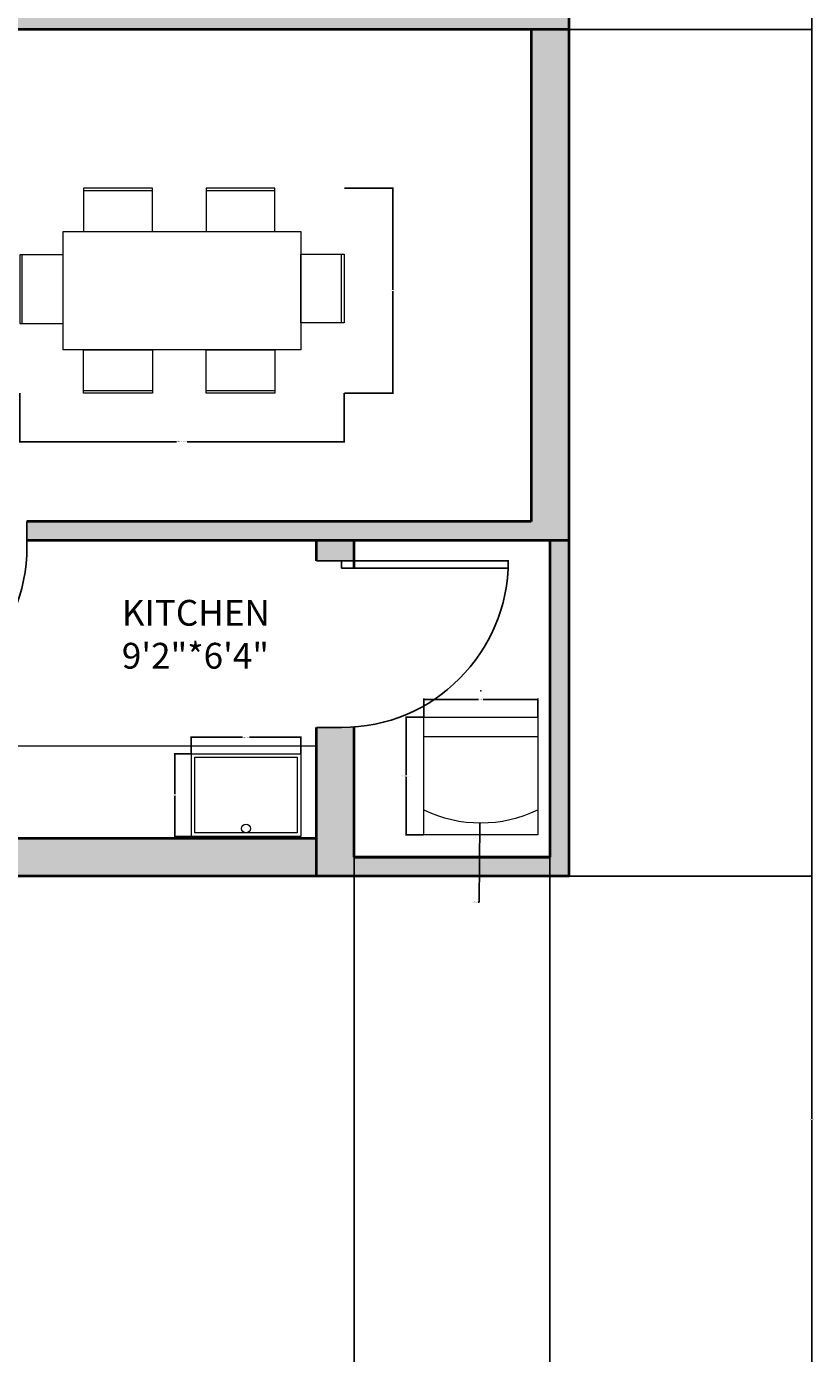
# Model space of a CAD drawing. Units: inches. Extents: x 1642 to 2399, y 1011 to 2291.
# Tile 6 of 7: x 2210 to 2399, y 1595 to 1913. Entities that reach past the tile are written whole.
import ezdxf

# ---------------------------------------------------------------- set-up
doc = ezdxf.new("R2010")
doc.units = ezdxf.units.IN
for name, color, linetype, lineweight in [('A-ANNO-DIMS', 2, 'Continuous', 18), ('A-AREA-IDEN', 7, 'Continuous', 20), ('A-DOOR', 4, 'Continuous', 25), ('A-EQPM', 8, 'Continuous', 18), ('A-FLOR-CASE', 30, 'Continuous', 18), ('A-FLOR-FIXT', 9, 'Continuous', 18), ('A-FURN', 8, 'Continuous', 18), ('A-WALL-PATT', 40, 'Continuous', 13), ('WALL', 40, 'Continuous', 40)]:
    doc.layers.add(name, color=color, linetype=linetype, lineweight=lineweight)
doc.styles.get("Standard").update_dxf_attribs({"font": 'arial.ttf'})
doc.dimstyles.get("Standard").update_dxf_attribs({"dimtxt": 0.18, "dimasz": 0.18, "dimexe": 0.18, "dimexo": 0.0625, "dimgap": 0.09, "dimtad": 0, "dimtih": 1, "dimtoh": 1, "dimdec": 4, "dimzin": 0, "dimdsep": 46, "dimtxsty": 'Standard', "dimcen": 0.09, "dimadec": 0, "dimazin": 0, "dimtfac": 1, "dimtdec": 4, "dimtofl": 0, "dimtmove": 0, "dimatfit": 3, "dimfxl": 1, "dimtolj": 1, "dimtzin": 0, "dimarcsym": 0})

# ---------------------------------------------------------------- blocks, each defined once
blk = doc.blocks.new('*U2')
for p, q in [((0, 0), (0, -6)), ((40, 0), (40, -6))]:
    blk.add_line(p, q)
blk.add_lwpolyline([(0, 0), (0, 40), (1.75, 40), (1.75, 0)], close=True)
blk.add_arc((0, 0), 40, 0, 90)
blk = doc.blocks.new('TABLE-DINING-SIX-SEAT')
for p, q in [((15.31, 48.55), (31.81, 48.55)), ((44.68, 48.55), (61.18, 48.55)), ((0.59, 16.67), (0.59, 33.17)), ((77.22, 16.83), (77.22, 33.33)), ((15.31, 0.59), (31.81, 0.59)), ((44.68, 0.59), (61.18, 0.59))]:
    blk.add_line(p, q)
for points in [[(15.31, 38.77), (31.81, 38.77), (31.81, 49.15), (15.31, 49.15)], [(44.68, 38.77), (61.18, 38.77), (61.18, 49.15), (44.68, 49.15)], [(10.38, 38.77), (67.43, 38.77), (67.43, 10.38), (10.38, 10.38)], [(10.38, 16.67), (10.38, 33.17), (0, 33.17), (0, 16.67)], [(67.43, 16.83), (67.43, 33.33), (77.81, 33.33), (77.81, 16.83)], [(15.31, 10.38), (31.81, 10.38), (31.81, 0), (15.31, 0)], [(44.68, 10.38), (61.18, 10.38), (61.18, 0), (44.68, 0)]]:
    blk.add_lwpolyline(points, close=True)
blk = doc.blocks.new('SINK-KITCHEN-SINGLE')
for points in [[(0, 19.82), (26.24, 19.82), (26.24, 0), (0, 0)], [(0.83, 18.98), (25.41, 18.98), (25.41, 0.83), (0.83, 0.83)]]:
    blk.add_lwpolyline(points, close=True)
blk.add_circle((13.12, 17.93), 1.05)
blk = doc.blocks.new('UTILITY-APPLIANCE')
blk.add_line((0, 4.7), (27.35, 4.7))
blk.add_lwpolyline([(0, 28.26), (27.35, 28.26), (27.35, 0), (0, 0)], close=True)
blk.add_arc((13.68, -6.28), 31.65, 64.3994, 115.6006)
blk = doc.blocks.new('*D18')
at = {"layer": 'A-ANNO-DIMS', "color": 0, "lineweight": -2, "transparency": 16777216}
for p, q in [((2208.46, 1825.25), (2208.46, 1813.46)), ((2286.28, 1825.25), (2286.28, 1813.46)), ((2208.64, 1813.64), (2246.09, 1813.64)), ((2286.1, 1813.64), (2248.65, 1813.64))]:
    blk.add_line(p, q, dxfattribs=at)
at = {"layer": 'A-ANNO-DIMS', "color": 0, "transparency": 16777216}
for points in [[(2208.64, 1813.67), (2208.64, 1813.61), (2208.46, 1813.64)], [(2286.1, 1813.67), (2286.1, 1813.61), (2286.28, 1813.64)]]:
    blk.add_solid(points, dxfattribs=at)
at = {"layer": 'Defpoints', "color": 0, "transparency": 16777216}
for p in [(2208.46, 1825.31), (2286.28, 1825.31), (2286.28, 1813.64)]:
    blk.add_point(p, dxfattribs=at)
at = {"layer": 'A-ANNO-DIMS', "color": 0, "transparency": 16777216, "insert": (2247.37, 1813.64), "char_height": 0.18, "attachment_point": 5}
blk.add_mtext('\\A1;DINING SET 78 TYP.', dxfattribs=at)
blk = doc.blocks.new('*D19')
at = {"layer": 'A-ANNO-DIMS', "color": 0, "lineweight": -2, "transparency": 16777216}
for p, q in [((2286.34, 1874.46), (2298.13, 1874.46)), ((2297.95, 1874.28), (2297.95, 1850.07)), ((2297.95, 1825.49), (2297.95, 1849.7)), ((2286.34, 1825.31), (2298.13, 1825.31))]:
    blk.add_line(p, q, dxfattribs=at)
at = {"layer": 'A-ANNO-DIMS', "color": 0, "transparency": 16777216}
for points in [[(2297.92, 1874.28), (2297.98, 1874.28), (2297.95, 1874.46)], [(2297.92, 1825.49), (2297.98, 1825.49), (2297.95, 1825.31)]]:
    blk.add_solid(points, dxfattribs=at)
at = {"layer": 'Defpoints', "color": 0, "transparency": 16777216}
for p in [(2286.28, 1874.46), (2297.95, 1874.46), (2286.28, 1825.31)]:
    blk.add_point(p, dxfattribs=at)
at = {"layer": 'A-ANNO-DIMS', "color": 0, "transparency": 16777216, "insert": (2297.95, 1849.88), "char_height": 0.18, "attachment_point": 5}
blk.add_mtext('\\A1;49 TYP.', dxfattribs=at)
blk = doc.blocks.new('*D24')
at = {"layer": 'A-ANNO-DIMS', "color": 0, "lineweight": -2, "transparency": 16777216}
for p, q in [((2249.62, 1738.86), (2249.62, 1742.91)), ((2249.8, 1742.73), (2261.89, 1742.73)), ((2275.69, 1742.73), (2263.6, 1742.73)), ((2275.87, 1738.86), (2275.87, 1742.91))]:
    blk.add_line(p, q, dxfattribs=at)
at = {"layer": 'A-ANNO-DIMS', "color": 0, "transparency": 16777216}
for points in [[(2249.8, 1742.76), (2249.8, 1742.7), (2249.62, 1742.73)], [(2275.69, 1742.76), (2275.69, 1742.7), (2275.87, 1742.73)]]:
    blk.add_solid(points, dxfattribs=at)
at = {"layer": 'Defpoints', "color": 0, "transparency": 16777216}
for p in [(2249.62, 1742.73), (2249.62, 1738.8), (2275.87, 1738.8)]:
    blk.add_point(p, dxfattribs=at)
at = {"layer": 'A-ANNO-DIMS', "color": 0, "transparency": 16777216, "insert": (2262.74, 1742.73), "char_height": 0.18, "attachment_point": 5}
blk.add_mtext('\\A1;SINK 26 TYP.', dxfattribs=at)
blk = doc.blocks.new('*D25')
at = {"layer": 'A-ANNO-DIMS', "color": 0, "lineweight": -2, "transparency": 16777216}
for p, q in [((2249.56, 1738.8), (2245.51, 1738.8)), ((2245.69, 1738.62), (2245.69, 1729.07)), ((2245.69, 1719.16), (2245.69, 1728.71)), ((2249.56, 1718.98), (2245.51, 1718.98))]:
    blk.add_line(p, q, dxfattribs=at)
at = {"layer": 'A-ANNO-DIMS', "color": 0, "transparency": 16777216}
for points in [[(2245.66, 1738.62), (2245.72, 1738.62), (2245.69, 1738.8)], [(2245.66, 1719.16), (2245.72, 1719.16), (2245.69, 1718.98)]]:
    blk.add_solid(points, dxfattribs=at)
at = {"layer": 'Defpoints', "color": 0, "transparency": 16777216}
for p in [(2249.62, 1738.8), (2245.69, 1718.98), (2249.62, 1718.98)]:
    blk.add_point(p, dxfattribs=at)
at = {"layer": 'A-ANNO-DIMS', "color": 0, "transparency": 16777216, "insert": (2245.69, 1728.89), "char_height": 0.18, "attachment_point": 5}
blk.add_mtext('\\A1;20 TYP.', dxfattribs=at)
blk = doc.blocks.new('*D26')
at = {"layer": 'A-ANNO-DIMS', "color": 0, "lineweight": -2, "transparency": 16777216}
for p, q in [((2305.36, 1747.59), (2301, 1747.59)), ((2301.18, 1747.41), (2301.18, 1733.64)), ((2301.18, 1719.51), (2301.18, 1733.28)), ((2305.36, 1719.33), (2301, 1719.33))]:
    blk.add_line(p, q, dxfattribs=at)
at = {"layer": 'A-ANNO-DIMS', "color": 0, "transparency": 16777216}
for points in [[(2301.15, 1747.41), (2301.21, 1747.41), (2301.18, 1747.59)], [(2301.15, 1719.51), (2301.21, 1719.51), (2301.18, 1719.33)]]:
    blk.add_solid(points, dxfattribs=at)
at = {"layer": 'Defpoints', "color": 0, "transparency": 16777216}
for p in [(2305.42, 1747.59), (2301.18, 1719.33), (2305.42, 1719.33)]:
    blk.add_point(p, dxfattribs=at)
at = {"layer": 'A-ANNO-DIMS', "color": 0, "transparency": 16777216, "insert": (2301.18, 1733.46), "char_height": 0.18, "attachment_point": 5}
blk.add_mtext('\\A1;APPLIANCE 28 TYP.', dxfattribs=at)
blk = doc.blocks.new('*D27')
at = {"layer": 'A-ANNO-DIMS', "color": 0, "lineweight": -2, "transparency": 16777216}
for p, q in [((2305.42, 1747.65), (2305.42, 1752.01)), ((2305.6, 1751.83), (2318.57, 1751.83)), ((2332.59, 1751.83), (2319.63, 1751.83)), ((2332.77, 1747.65), (2332.77, 1752.01))]:
    blk.add_line(p, q, dxfattribs=at)
at = {"layer": 'A-ANNO-DIMS', "color": 0, "transparency": 16777216}
for points in [[(2305.6, 1751.86), (2305.6, 1751.8), (2305.42, 1751.83)], [(2332.59, 1751.86), (2332.59, 1751.8), (2332.77, 1751.83)]]:
    blk.add_solid(points, dxfattribs=at)
at = {"layer": 'Defpoints', "color": 0, "transparency": 16777216}
for p in [(2305.42, 1751.83), (2305.42, 1747.59), (2332.77, 1747.59)]:
    blk.add_point(p, dxfattribs=at)
at = {"layer": 'A-ANNO-DIMS', "color": 0, "transparency": 16777216, "insert": (2319.1, 1751.83), "char_height": 0.18, "attachment_point": 5}
blk.add_mtext('\\A1;27 TYP.', dxfattribs=at)
blk = doc.blocks.new('*D36')
at = {"layer": 'A-ANNO-DIMS', "color": 0, "lineweight": -2, "transparency": 16777216}
for p, q in [((2340.24, 1709.46), (2398.73, 1709.46)), ((2398.55, 1709.28), (2398.55, 1651.26)), ((2398.55, 1592.89), (2398.55, 1650.9)), ((2340.24, 1592.71), (2398.73, 1592.71))]:
    blk.add_line(p, q, dxfattribs=at)
at = {"layer": 'A-ANNO-DIMS', "color": 0, "transparency": 16777216}
for points in [[(2398.52, 1709.28), (2398.58, 1709.28), (2398.55, 1709.46)], [(2398.52, 1592.89), (2398.58, 1592.89), (2398.55, 1592.71)]]:
    blk.add_solid(points, dxfattribs=at)
at = {"layer": 'Defpoints', "color": 0, "transparency": 16777216}
for p in [(2340.18, 1709.46), (2398.55, 1709.46), (2340.18, 1592.71)]:
    blk.add_point(p, dxfattribs=at)
at = {"layer": 'A-ANNO-DIMS', "color": 0, "transparency": 16777216, "insert": (2398.55, 1651.08), "char_height": 0.18, "attachment_point": 5}
blk.add_mtext('\\A1;116.75', dxfattribs=at)
blk = doc.blocks.new('*D37')
at = {"layer": 'A-ANNO-DIMS', "color": 0, "lineweight": -2, "transparency": 16777216}
for p, q in [((2340.27, 2232.46), (2398.73, 2232.46)), ((2398.55, 2232.28), (2398.55, 1971.14)), ((2398.55, 1709.64), (2398.55, 1970.77)), ((2340.24, 1709.46), (2398.73, 1709.46))]:
    blk.add_line(p, q, dxfattribs=at)
at = {"layer": 'A-ANNO-DIMS', "color": 0, "transparency": 16777216}
for points in [[(2398.52, 2232.28), (2398.58, 2232.28), (2398.55, 2232.46)], [(2398.52, 1709.64), (2398.58, 1709.64), (2398.55, 1709.46)]]:
    blk.add_solid(points, dxfattribs=at)
at = {"layer": 'Defpoints', "color": 0, "transparency": 16777216}
for p in [(2340.21, 2232.46), (2398.55, 2232.46), (2340.18, 1709.46)]:
    blk.add_point(p, dxfattribs=at)
at = {"layer": 'A-ANNO-DIMS', "color": 0, "transparency": 16777216, "insert": (2398.55, 1970.96), "char_height": 0.18, "attachment_point": 5}
blk.add_mtext('\\A1;523', dxfattribs=at)
blk = doc.blocks.new('*D38')
at = {"layer": 'A-ANNO-DIMS', "color": 0, "lineweight": -2, "transparency": 16777216}
for p, q in [((2340.27, 1912.46), (2398.73, 1912.46)), ((2398.55, 1912.28), (2398.55, 1811.14)), ((2398.55, 1709.64), (2398.55, 1810.77)), ((2340.24, 1709.46), (2398.73, 1709.46))]:
    blk.add_line(p, q, dxfattribs=at)
at = {"layer": 'A-ANNO-DIMS', "color": 0, "transparency": 16777216}
for points in [[(2398.52, 1912.28), (2398.58, 1912.28), (2398.55, 1912.46)], [(2398.52, 1709.64), (2398.58, 1709.64), (2398.55, 1709.46)]]:
    blk.add_solid(points, dxfattribs=at)
at = {"layer": 'Defpoints', "color": 0, "transparency": 16777216}
for p in [(2340.21, 1912.46), (2398.55, 1912.46), (2340.18, 1709.46)]:
    blk.add_point(p, dxfattribs=at)
at = {"layer": 'A-ANNO-DIMS', "color": 0, "transparency": 16777216, "insert": (2398.55, 1810.96), "char_height": 0.18, "attachment_point": 5}
blk.add_mtext('\\A1;203', dxfattribs=at)
blk = doc.blocks.new('*D47')
at = {"layer": 'A-ANNO-DIMS', "color": 0, "lineweight": -2, "transparency": 16777216}
for p, q in [((2288.68, 1713.89), (2288.68, 1011.19)), ((2335.68, 1713.89), (2335.68, 1011.19)), ((2288.86, 1011.37), (2311.96, 1011.37)), ((2335.5, 1011.37), (2312.4, 1011.37))]:
    blk.add_line(p, q, dxfattribs=at)
at = {"layer": 'A-ANNO-DIMS', "color": 0, "transparency": 16777216}
for points in [[(2288.86, 1011.4), (2288.86, 1011.34), (2288.68, 1011.37)], [(2335.5, 1011.4), (2335.5, 1011.34), (2335.68, 1011.37)]]:
    blk.add_solid(points, dxfattribs=at)
at = {"layer": 'Defpoints', "color": 0, "transparency": 16777216}
for p in [(2288.68, 1713.96), (2335.68, 1713.96), (2335.68, 1011.37)]:
    blk.add_point(p, dxfattribs=at)
at = {"layer": 'A-ANNO-DIMS', "color": 0, "transparency": 16777216, "insert": (2312.18, 1011.37), "char_height": 0.18, "attachment_point": 5}
blk.add_mtext('\\A1;47', dxfattribs=at)
blk = doc.blocks.new('*D56')
at = {"layer": 'A-ANNO-DIMS', "color": 0, "lineweight": -2, "transparency": 16777216}
for p, q in [((2319.01, 1753.87), (2319.19, 1753.87)), ((2319.1, 1753.78), (2319.1, 1753.96)), ((2318.66, 1703.22), (2318.82, 1722.03)), ((2318.48, 1703.22), (2318.66, 1703.22))]:
    blk.add_line(p, q, dxfattribs=at)
at = {"layer": 'A-ANNO-DIMS', "color": 0, "transparency": 16777216}
blk.add_solid([(2318.79, 1722.03), (2318.85, 1722.03), (2318.82, 1722.21)], dxfattribs=at)
at = {"layer": 'Defpoints', "color": 0, "transparency": 16777216}
for p in [(2319.1, 1753.87), (2318.82, 1722.21)]:
    blk.add_point(p, dxfattribs=at)
at = {"layer": 'A-ANNO-DIMS', "color": 0, "transparency": 16777216, "insert": (2317.74, 1703.22), "char_height": 0.18, "attachment_point": 5}
blk.add_mtext('\\A1;4X R31.654', dxfattribs=at)

msp = doc.modelspace()

# ---------------------------------------------------------------- hatches: boundary and pattern name
at = {"layer": 'A-WALL-PATT'}
h = msp.add_hatch(color=256, dxfattribs=at)
h.dxf.hatch_style = 1
h.paths.add_polyline_path([(2340.1804, 2185.4562), (2211.0983, 2185.4562, -0.01876983), (2211.211, 2182.4562), (2211.211, 2176.4562), (2331.211, 2176.4562), (2331.211, 2043.4562), (2171.211, 2043.4562), (2171.211, 2038.9562), (2331.211, 2038.9562), (2331.211, 1916.9562), (2171.211, 1916.9562), (2171.211, 1918.9365), (2166.711, 1918.9365), (2166.711, 1912.4562), (2340.1804, 1912.4562)])
h.paths.add_polyline_path([(2171.211, 2043.4562), (2171.211, 2043.9025), (2170.5217, 2043.9025), (2166.711, 2043.9025), (2166.711, 2038.9562), (2166.711, 1958.9365), (2171.211, 1958.9365)], flags=17)
h.paths.add_polyline_path([(2129.211, 1971.5979), (2124.711, 1971.5979), (2124.711, 1918.4562), (2067.711, 1918.4562), (2067.711, 1913.9562), (2129.211, 1913.9562)])
h.paths.add_polyline_path([(2067.711, 2015.4562), (2124.711, 2015.4562), (2124.711, 2019.9562), (2058.711, 2019.9562), (2058.711, 2015.4562), (2058.711, 1922.9562), (1982.211, 1922.9562), (1982.211, 2015.4562), (1982.211, 2019.9562), (1916.211, 2019.9562), (1916.211, 2070.9562), (1911.711, 2070.9562), (1911.711, 2015.4562), (1911.711, 2012.302), (1916.211, 2012.302), (1916.211, 2015.4562), (1973.211, 2015.4562), (1973.211, 1918.4562), (1973.211, 1913.9562), (2017.1804, 1913.9562), (2067.711, 1913.9562), (2067.711, 1918.4562)])
h.paths.add_polyline_path([(2131.1386, 2075.4562), (2118.1934, 2075.4562), (2118.1934, 2070.9562), (2131.1386, 2070.9562)], flags=17)
h.paths.add_polyline_path([(1918.8034, 2075.4562), (1909.4956, 2075.4562), (1909.4956, 2070.9562), (1918.8034, 2070.9562)], flags=17)
h.paths.add_polyline_path([(1874.211, 2029.9562), (1869.711, 2029.9562), (1869.711, 1960.7404), (1874.211, 1960.7404)], flags=17)
h.paths.add_polyline_path([(1916.211, 1972.302), (1911.711, 1972.302), (1911.711, 1918.4562), (1916.211, 1918.4562)], flags=17)
h.paths.add_polyline_path([(2340.1804, 1912.4562), (2331.1804, 1912.4562), (2331.1804, 1794.4562), (2210.1804, 1794.4562), (2210.1804, 1789.9562), (2279.6804, 1789.9562), (2340.1804, 1789.9562)])
h.paths.add_polyline_path([(2288.6804, 1789.9562), (2279.6804, 1789.9562), (2279.6804, 1785.0846), (2285.6804, 1785.0846), (2288.6804, 1785.0846)], flags=17)
h.paths.add_polyline_path([(2169.6804, 1789.9562), (2170.1804, 1789.9562), (2170.1804, 1794.4562), (2165.1804, 1794.4562), (2165.1804, 1713.9562), (2165.1804, 1709.4562), (2279.6804, 1709.4562), (2279.6804, 1718.4562), (2169.6804, 1718.4562)])
h.paths.add_polyline_path([(2288.6804, 1745.1973, -0.01876983), (2285.6804, 1745.0846), (2279.6804, 1745.0846), (2279.6804, 1709.4562), (2340.1804, 1709.4562), (2340.1804, 1789.9562), (2335.6804, 1789.9562), (2335.6804, 1713.9562), (2288.6804, 1713.9562)])
h.paths.add_polyline_path([(2165.1804, 1713.9562), (2140.6229, 1713.9562), (2088.923, 1713.9562), (2069.7509, 1713.9562), (2060.4457, 1713.9562), (2060.4457, 1709.4562), (2165.1804, 1709.4562)])
h.paths.add_polyline_path([(2020.4457, 1713.9562), (2017.1804, 1713.9562), (2012.6804, 1713.9562), (2009.1946, 1713.9562), (2009.1946, 1709.4562), (2020.4457, 1709.4562)])
h.paths.add_polyline_path([(1969.1946, 1713.9562), (1864.6804, 1713.9562), (1864.6804, 1798.9562), (1860.1804, 1798.9562), (1860.1804, 1792.9562), (1860.1804, 1752.9562), (1860.1804, 1718.4562), (1750.1804, 1718.4562), (1750.1804, 1749.2419), (1744.1804, 1749.2419, -0.01876983), (1741.1804, 1749.3546), (1741.1804, 1709.4562), (1969.1946, 1709.4562)])
h.paths.add_polyline_path([(1741.1804, 1803.4562), (1700.711, 1803.4562), (1700.711, 1794.4562), (1741.1804, 1794.4562)])
h.paths.add_polyline_path([(1820.1804, 1798.9562), (1741.1804, 1798.9562), (1741.1804, 1794.4562), (1741.1804, 1790.0365), (1741.1804, 1789.2419), (1744.1804, 1789.2419), (1750.1804, 1789.2419), (1750.1804, 1794.4562), (1820.1804, 1794.4562)], flags=17)
h.paths.add_polyline_path([(1800.6804, 1709.4562), (1796.1804, 1709.4562), (1796.1804, 1592.7078), (1978.9325, 1592.7078), (1978.9325, 1597.2078), (1800.6804, 1597.2078)])
h.paths.add_polyline_path([(2097.0678, 1709.4562), (2088.0678, 1709.4562), (2088.0678, 1599.6874), (2088.0678, 1597.2078), (2097.0678, 1597.2078)], flags=17)
h.paths.add_polyline_path([(2186.8766, 1709.4562), (2182.3766, 1709.4562), (2182.3766, 1597.2078), (2071.4624, 1597.2078), (2071.4624, 1592.7078), (2186.8766, 1592.7078)])
h.paths.add_polyline_path([(2078.1934, 2075.4562), (2022.711, 2075.4562), (2022.711, 2223.4562), (2166.711, 2223.4562), (2166.711, 2075.4562), (2166.711, 2070.9562), (2171.211, 2070.9562), (2171.211, 2138.8919), (2171.211, 2227.9562), (2335.711, 2227.9562), (2335.711, 2185.4562), (2340.1804, 2185.4562), (2340.1804, 2232.4562), (1874.211, 2232.4562), (1874.211, 2223.4562), (2018.211, 2223.4562), (2018.211, 2075.4562), (1958.8034, 2075.4562), (1958.8034, 2070.9562), (2018.211, 2070.9562), (2018.211, 2019.9562), (1982.211, 2019.9562), (1982.211, 2015.4562), (1982.211, 2010.9562), (2058.711, 2010.9562), (2058.711, 2015.4562), (2058.711, 2019.9562), (2022.711, 2019.9562), (2022.711, 2070.9562), (2078.1934, 2070.9562)])
h.paths.add_polyline_path([(1874.211, 2171.9562), (1874.211, 2176.4562), (1861.9371, 2176.4562), (1861.9371, 2173.4562), (1861.9371, 2167.4562), (1869.711, 2167.4562), (1869.711, 2069.7602), (1874.211, 2069.7602)], flags=17)
h.paths.add_polyline_path([(1705.211, 2227.9562), (1865.211, 2227.9562), (1865.211, 2176.4562), (1874.211, 2176.4562), (1874.211, 2232.4562), (1700.711, 2232.4562), (1700.711, 2176.4562), (1705.211, 2176.4562)])
h.paths.add_polyline_path([(1709.711, 2167.4562), (1821.9371, 2167.4562), (1821.9371, 2173.4562, -0.01876983), (1822.0498, 2176.4562), (1700.711, 2176.4562), (1700.711, 1913.9562), (1860.1804, 1913.9562), (1864.6804, 1913.9562), (1973.211, 1913.9562), (1973.211, 1918.4562), (1916.211, 1918.4562), (1874.211, 1918.4562), (1874.211, 1920.7404), (1869.711, 1920.7404), (1869.711, 1918.4562), (1860.1804, 1918.4562), (1709.711, 1918.4562), (1709.711, 2029.9562), (1874.211, 2029.9562), (1874.211, 2037.0364), (1869.711, 2037.0364), (1869.711, 2034.4562), (1709.711, 2034.4562)])
h.paths.add_polyline_path([(2017.1804, 1913.9562), (2012.6804, 1913.9562), (2012.6804, 1713.9562), (2017.1804, 1713.9562)])
h.paths.add_polyline_path([(1952.4341, 2110.3716), (2000.4134, 2110.3716), (2000.4134, 2133.4189), (1952.4341, 2133.4189)], flags=25)
h.paths.add_polyline_path([(2042.3983, 2110.7121), (2090.3775, 2110.7121), (2090.3775, 2133.7594), (2042.3983, 2133.7594)], flags=25)
h.paths.add_polyline_path([(2201.7332, 2091.8715), (2249.7125, 2091.8715), (2249.7125, 2114.9188), (2201.7332, 2114.9188)], flags=25)
h.paths.add_polyline_path([(1805.186, 2077.6915), (1853.1653, 2077.6915), (1853.1653, 2100.7388), (1805.186, 2100.7388)], flags=25)
h.paths.add_polyline_path([(1794.8897, 1974.6584), (1842.869, 1974.6584), (1842.869, 1997.7057), (1794.8897, 1997.7057)], flags=25)
h.paths.add_polyline_path([(2229.1796, 2204.4209), (2315.1362, 2204.4209), (2315.1362, 2217.1488), (2229.1796, 2217.1488)], flags=25)
h.paths.add_polyline_path([(1715.2159, 2199.5328), (1801.1724, 2199.5328), (1801.1724, 2212.2607), (1715.2159, 2212.2607)], flags=25)
h.paths.add_polyline_path([(2230.7681, 1755.7109), (2271.7283, 1755.7109), (2271.7283, 1778.7582), (2230.7681, 1778.7582)], flags=25)
h.paths.add_polyline_path([(1763.4713, 1764.1742), (1804.4315, 1764.1742), (1804.4315, 1787.2215), (1763.4713, 1787.2215)], flags=25)
h.paths.add_polyline_path([(2076.2643, 1955.0495), (2111.326, 1955.0495), (2111.326, 1978.0968), (2076.2643, 1978.0968)], flags=25)
h.paths.add_polyline_path([(1932.854, 1956.1217), (1967.9158, 1956.1217), (1967.9158, 1979.169), (1932.854, 1979.169)], flags=25)
h.paths.add_polyline_path([(2048.1203, 2031.6107), (2083.1821, 2031.6107), (2083.1821, 2054.658), (2048.1203, 2054.658)], flags=25)
h.paths.add_polyline_path([(2163.5754, 1863.7569), (2208.2347, 1863.7569), (2208.2347, 1886.8042), (2163.5754, 1886.8042)], flags=9)
h.paths.add_polyline_path([(2039.9286, 1809.0957), (2084.5879, 1809.0957), (2084.5879, 1832.143), (2039.9286, 1832.143)], flags=9)
h.paths.add_polyline_path([(1901.0045, 1814.0452), (1945.6638, 1814.0452), (1945.6638, 1837.0925), (1901.0045, 1837.0925)], flags=9)
h.paths.add_polyline_path([(1833.7282, 1852.5627), (1878.3875, 1852.5627), (1878.3875, 1875.61), (1833.7282, 1875.61)], flags=9)
h.paths.add_polyline_path([(2219.1375, 1926.2139), (2267.1167, 1926.2139), (2267.1167, 1949.2612), (2219.1375, 1949.2612)], flags=25)
h.paths.add_polyline_path([(1956.9598, 2029.7735), (1992.0216, 2029.7735), (1992.0216, 2052.8208), (1956.9598, 2052.8208)], flags=25)
h.paths.add_polyline_path([(2229.3, 1523.3399), (2270.2602, 1523.3399), (2270.2602, 1546.3872), (2229.3, 1546.3872)], flags=9)
h.paths.add_polyline_path([(1772.3039, 1526.9922), (1813.2641, 1526.9922), (1813.2641, 1550.0394), (1772.3039, 1550.0394)], flags=9)
h.paths.add_polyline_path([(2172.587, 1420.6999), (2217.2463, 1420.6999), (2217.2463, 1443.7472), (2172.587, 1443.7472)], flags=9)
h.paths.add_polyline_path([(1814.3549, 1422.215), (1859.0143, 1422.215), (1859.0143, 1445.2623), (1814.3549, 1445.2623)], flags=9)
h.paths.add_polyline_path([(2186.0372, 1305.6227), (2234.0165, 1305.6227), (2234.0165, 1328.67), (2186.0372, 1328.67)], flags=9)
h.paths.add_polyline_path([(1756.747, 1349.0694), (1804.7263, 1349.0694), (1804.7263, 1372.1167), (1756.747, 1372.1167)], flags=9)
h.paths.add_polyline_path([(2239.449, 1214.6184), (2287.4282, 1214.6184), (2287.4282, 1237.6657), (2239.449, 1237.6657)], flags=9)
h.paths.add_polyline_path([(1767.104, 1213.8348), (1815.0832, 1213.8348), (1815.0832, 1236.8821), (1767.104, 1236.8821)], flags=9)
h.paths.add_polyline_path([(2046.6809, 1183.6854), (2094.6602, 1183.6854), (2094.6602, 1206.7327), (2046.6809, 1206.7327)], flags=9)
h.paths.add_polyline_path([(1947.2155, 1183.6854), (1995.1948, 1183.6854), (1995.1948, 1206.7327), (1947.2155, 1206.7327)], flags=9)
h.paths.add_polyline_path([(1959.3556, 1258.7871), (1994.4174, 1258.7871), (1994.4174, 1281.8344), (1959.3556, 1281.8344)], flags=9)
h.paths.add_polyline_path([(2049.6419, 1248.9629), (2084.7036, 1248.9629), (2084.7036, 1272.0102), (2049.6419, 1272.0102)], flags=9)
h.paths.add_polyline_path([(2092.7532, 1327.4852), (2127.815, 1327.4852), (2127.815, 1350.5325), (2092.7532, 1350.5325)], flags=9)
h.paths.add_polyline_path([(1944.9358, 1327.4852), (1979.9976, 1327.4852), (1979.9976, 1350.5325), (1944.9358, 1350.5325)], flags=9)
h.paths.add_polyline_path([(1974.5055, 1650.063), (2006.3695, 1650.063), (2006.3695, 1662.7909), (1974.5055, 1662.7909)], flags=9)

# ---------------------------------------------------------------- linework, layer by layer
at = {"layer": 'A-FLOR-CASE'}
msp.add_line((2279.6804, 1740.5928), (2169.6804, 1740.5928), dxfattribs=at)
at = {"layer": 'WALL'}
for p, q in [((2340.211, 2038.9562), (2340.211, 1912.4562)), ((2340.211, 1912.4562), (2166.711, 1912.4562)), ((2331.1804, 1912.4562), (2331.1804, 1794.4562)), ((2340.1804, 1912.4562), (2340.1804, 1789.9562)), ((2331.1804, 1794.4562), (2210.1804, 1794.4562)), ((2340.1804, 1789.9562), (2210.1804, 1789.9562)), ((2279.6804, 1789.9562), (2210.1804, 1789.9562)), ((2279.6804, 1785.0846), (2279.6804, 1789.9562)), ((2288.6804, 1783.3346), (2288.6804, 1789.9562)), ((2340.1804, 1789.9562), (2335.6804, 1789.9562)), ((2335.6804, 1789.9562), (2335.6804, 1713.9562)), ((2340.1804, 1789.9562), (2340.1804, 1709.4562)), ((2279.6804, 1709.4562), (2279.6804, 1745.0846)), ((2288.6804, 1713.9562), (2288.6804, 1745.1973)), ((2279.6804, 1718.4562), (2169.6804, 1718.4562)), ((2335.6804, 1713.9562), (2288.6804, 1713.9562)), ((2288.6804, 1713.9562), (2335.6804, 1713.9562)), ((2279.6804, 1709.4562), (2165.1804, 1709.4562)), ((2340.1804, 1709.4562), (2279.6804, 1709.4562))]:
    msp.add_line(p, q, dxfattribs=at)
msp.add_lwpolyline([(1969.1946, 1709.4562), (1700.711, 1709.4562), (1700.711, 2232.4562), (2340.1804, 2232.4562), (2340.1804, 1709.4562), (2060.4457, 1709.4562)], dxfattribs=at)

# ---------------------------------------------------------------- block references
at = {"layer": 'A-DOOR', "xscale": -1, "rotation": 180}
msp.add_blockref('*U2', (2170.1804, 1788.4562), dxfattribs=at)
at = {"layer": 'A-DOOR', "rotation": 270}
msp.add_blockref('*U2', (2285.6804, 1785.0846), dxfattribs=at)
at = {"layer": 'A-EQPM', "rotation": 180}
msp.add_blockref('UTILITY-APPLIANCE', (2332.7735, 1747.589), dxfattribs=at)
at = {"layer": 'A-FLOR-FIXT', "rotation": 180}
msp.add_blockref('SINK-KITCHEN-SINGLE', (2275.8657, 1738.7959), dxfattribs=at)
at = {"layer": 'A-FURN'}
msp.add_blockref('TABLE-DINING-SIX-SEAT', (2208.4629, 1825.31), dxfattribs=at)

# ---------------------------------------------------------------- texts
at = {"layer": 'A-AREA-IDEN', "insert": (2232.9442, 1775.6848), "char_height": 6.17647, "attachment_point": 1}
msp.add_mtext_dynamic_manual_height_columns('KITCHEN\\P9\'2"*6\'4"', width=136.850471, gutter_width=30.8823, heights=[0], dxfattribs=at)

# ---------------------------------------------------------------- dimensions: what is measured, and where the dimension line sits
at = {"layer": 'A-ANNO-DIMS'}
for base, p1, p2, override, picture, middle in [((2398.551, 2232.4562), (2340.1804, 1709.4562), (2340.211, 2232.4562), {"dimdec": 0, "dimlfac": 1, "dimrnd": 0, "dimzin": 0, "dimdsep": 46, "dimlunit": 2}, '*D37', (2398.551, 1970.9562)), ((2398.551, 1912.4562), (2340.1804, 1709.4562), (2340.211, 1912.4562), {"dimdec": 0, "dimlfac": 1, "dimrnd": 0, "dimzin": 0, "dimdsep": 46, "dimlunit": 2}, '*D38', (2398.551, 1810.9562)), ((2398.551, 1709.4562), (2340.1804, 1592.7078), (2340.1804, 1709.4562), {"dimdec": 2, "dimlfac": 1, "dimrnd": 0, "dimzin": 0, "dimdsep": 46, "dimlunit": 2}, '*D36', (2398.551, 1651.082))]:
    dim = msp.add_linear_dim(base=base, p1=p1, p2=p2, angle=90, dimstyle='Standard', override=override, dxfattribs=at)
    dim.commit()
    dim.dimension.update_dxf_attribs({"geometry": picture, "text_midpoint": middle})
for base, p1, p2, angle, text, picture, middle in [((2297.9488, 1874.4579), (2286.2767, 1825.31), (2286.2767, 1874.4579), 90, '<> TYP.', '*D19', (2297.9488, 1849.8839)), ((2305.4187, 1751.8282), (2332.7735, 1747.589), (2305.4187, 1747.589), 180, '<> TYP.', '*D27', (2319.0961, 1751.8282)), ((2301.1796, 1719.3282), (2305.4187, 1747.589), (2305.4187, 1719.3282), 270, 'APPLIANCE <> TYP.', '*D26', (2301.1796, 1733.4586)), ((2249.6226, 1742.7324), (2275.8657, 1738.7959), (2249.6226, 1738.7959), 180, 'SINK <> TYP.', '*D24', (2262.7442, 1742.7324)), ((2245.6862, 1718.98), (2249.6226, 1738.7959), (2249.6226, 1718.98), 270, '<> TYP.', '*D25', (2245.6862, 1728.888))]:
    dim = msp.add_linear_dim(base=base, p1=p1, p2=p2, angle=angle, text=text, dimstyle='Standard', override={"dimdec": 0, "dimlfac": 1, "dimrnd": 0, "dimzin": 0, "dimdsep": 46, "dimlunit": 2}, dxfattribs=at)
    dim.commit()
    dim.dimension.update_dxf_attribs({"geometry": picture, "text_midpoint": middle})
dim = msp.add_linear_dim(base=(2286.2767, 1813.6379), p1=(2208.4629, 1825.31), p2=(2286.2767, 1825.31), text='DINING SET <> TYP.', dimstyle='Standard', override={"dimdec": 0, "dimlfac": 1, "dimrnd": 0, "dimzin": 0, "dimdsep": 46, "dimlunit": 2}, dxfattribs=at)
dim.commit()
dim.dimension.update_dxf_attribs({"geometry": '*D18', "text_midpoint": (2247.3698, 1813.6379)})
dim = msp.add_radius_dim(center=(2319.0961, 1753.8652), mpoint=(2318.825, 1722.2128), text='4X <>', dimstyle='Standard', override={"dimdec": 3, "dimlfac": 1, "dimrnd": 0, "dimzin": 0, "dimdsep": 46, "dimlunit": 2}, dxfattribs=at)
dim.commit()
dim.dimension.update_dxf_attribs({"geometry": '*D56', "text_midpoint": (2317.7358, 1703.2213), "dimtype": 164})
dim = msp.add_linear_dim(base=(2335.6804, 1011.3678), p1=(2288.6804, 1713.9562), p2=(2335.6804, 1713.9562), dimstyle='Standard', override={"dimdec": 0, "dimlfac": 1, "dimrnd": 0, "dimzin": 0, "dimdsep": 46, "dimlunit": 2}, dxfattribs=at)
dim.commit()
dim.dimension.update_dxf_attribs({"geometry": '*D47', "text_midpoint": (2312.1804, 1011.3678)})

doc.saveas('drawing.dxf')
